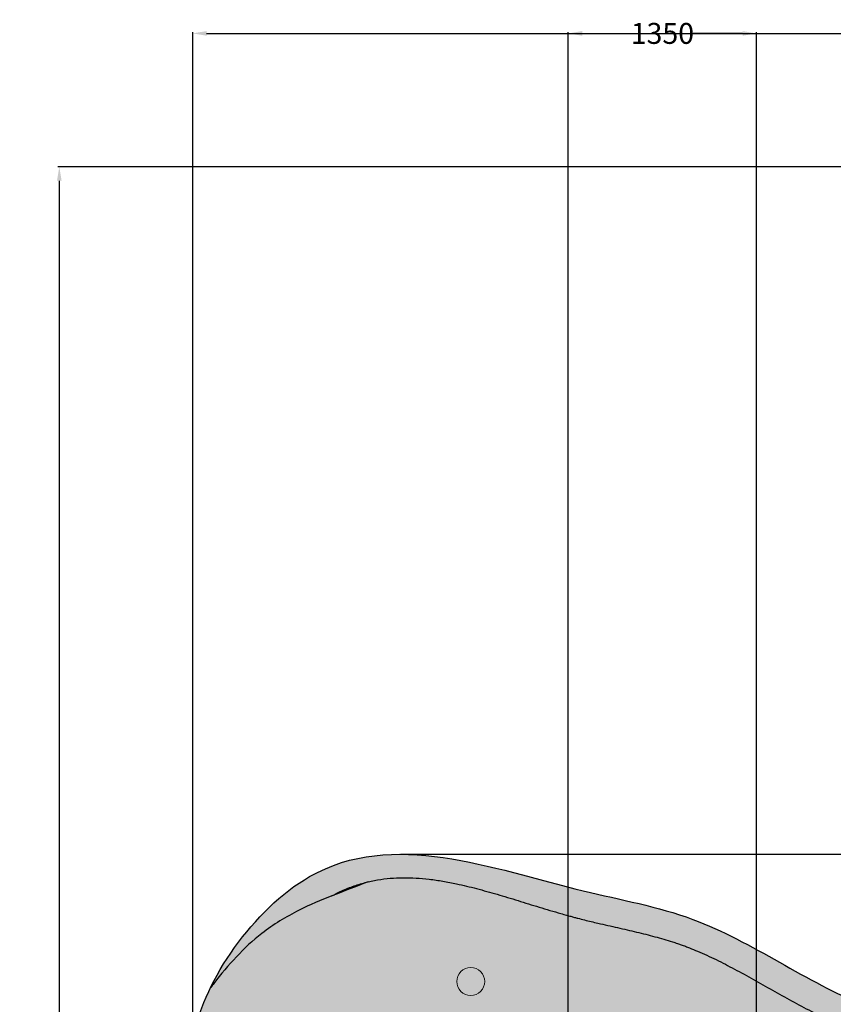
# Model space of a CAD drawing. Units: millimetres. Extents: x 11032 to 26788, y 3406 to 24505.
# Tile 75 of 78: x 11061 to 16895, y 17443 to 24505. Entities that reach past the tile are written whole.
import ezdxf

# ---------------------------------------------------------------- set-up
doc = ezdxf.new("R2010")
doc.units = ezdxf.units.MM
doc.header["$MEASUREMENT"] = 0
for name, color, linetype, lineweight in [('A-ANNO-DIMS', 2, 'Continuous', 18), ('A-ROOF', 7, 'Continuous', 30), ('E-LITE', 7, 'Continuous', 18), ('E-LITE-PATT', 7, 'Continuous', 13)]:
    doc.layers.add(name, color=color, linetype=linetype, lineweight=lineweight)
doc.layers.add('A-ROOF-PATT', color=9, linetype='Continuous', lineweight=13, true_color=0xc7c8ca)
doc.styles.get("Standard").update_dxf_attribs({"font": 'arial.ttf'})
doc.dimstyles.get("Standard").update_dxf_attribs({"dimtxt": 150, "dimasz": 100, "dimexe": 10, "dimexo": 5, "dimgap": 5, "dimtad": 0, "dimtih": 1, "dimtoh": 1, "dimdec": 0, "dimzin": 0, "dimdsep": 46, "dimtxsty": 'Standard', "dimcen": 0.09, "dimadec": 0, "dimazin": 0, "dimtfac": 1, "dimtdec": 0, "dimtofl": 0, "dimtmove": 0, "dimatfit": 3, "dimfxl": 1, "dimtolj": 1, "dimtzin": 0, "dimarcsym": 0})

# ---------------------------------------------------------------- blocks, each defined once
blk = doc.blocks.new('RECESSED-LIGHT-200')
blk.add_circle((100, 100), 100)
blk = doc.blocks.new('*D24')
at = {"layer": 'A-ANNO-DIMS', "color": 0, "lineweight": -2, "transparency": 16777216}
for p, q in [((13210.2, 17163), (13110.2, 17163)), ((13310.2, 17138), (13310.2, 17173)), ((13510.2, 17138), (13510.2, 17173)), ((13610.2, 17163), (13710.2, 17163))]:
    blk.add_line(p, q, dxfattribs=at)
at = {"layer": 'A-ANNO-DIMS', "color": 0, "transparency": 16777216}
for points in [[(13210.2, 17179.6), (13210.2, 17146.3), (13310.2, 17163)], [(13610.2, 17179.6), (13610.2, 17146.3), (13510.2, 17163)]]:
    blk.add_solid(points, dxfattribs=at)
at = {"layer": 'Defpoints', "color": 0, "transparency": 16777216}
for p in [(13510.2, 17163), (13310.2, 17133), (13510.2, 17133)]:
    blk.add_point(p, dxfattribs=at)
at = {"layer": 'A-ANNO-DIMS', "color": 0, "transparency": 16777216, "insert": (15077.8, 17163), "char_height": 150, "attachment_point": 5}
blk.add_mtext('\\A1;RECESSED LIGHT 200 TYP.', dxfattribs=at)
blk = doc.blocks.new('*D36')
at = {"layer": 'A-ANNO-DIMS', "color": 0, "lineweight": -2, "transparency": 16777216}
for p, q in [((12301.3, 17115.9), (12301.3, 24416.9)), ((12401.3, 24406.9), (18569.2, 24406.9)), ((25297.4, 24406.9), (19129.5, 24406.9)), ((25397.4, 4466.4), (25397.4, 24416.9))]:
    blk.add_line(p, q, dxfattribs=at)
at = {"layer": 'A-ANNO-DIMS', "color": 0, "transparency": 16777216}
for points in [[(12401.3, 24423.5), (12401.3, 24390.2), (12301.3, 24406.9)], [(25297.4, 24423.5), (25297.4, 24390.2), (25397.4, 24406.9)]]:
    blk.add_solid(points, dxfattribs=at)
at = {"layer": 'Defpoints', "color": 0, "transparency": 16777216}
for p in [(25397.4, 24406.9), (12301.3, 17110.9), (25397.4, 4461.4)]:
    blk.add_point(p, dxfattribs=at)
at = {"layer": 'A-ANNO-DIMS', "color": 0, "transparency": 16777216, "insert": (18849.3, 24406.9), "char_height": 150, "attachment_point": 5}
blk.add_mtext('\\A1;13096', dxfattribs=at)
blk = doc.blocks.new('*D37')
at = {"layer": 'A-ANNO-DIMS', "color": 0, "lineweight": -2, "transparency": 16777216}
for p, q in [((18087.7, 23450.4), (11334.8, 23450.4)), ((11344.8, 23350.4), (11344.8, 14037.5)), ((11344.8, 4561.4), (11344.8, 13874.3)), ((12927.7, 4461.4), (11334.8, 4461.4))]:
    blk.add_line(p, q, dxfattribs=at)
at = {"layer": 'A-ANNO-DIMS', "color": 0, "transparency": 16777216}
for points in [[(11328.1, 23350.4), (11361.4, 23350.4), (11344.8, 23450.4)], [(11328.1, 4561.4), (11361.4, 4561.4), (11344.8, 4461.4)]]:
    blk.add_solid(points, dxfattribs=at)
at = {"layer": 'Defpoints', "color": 0, "transparency": 16777216}
for p in [(11344.8, 23450.4), (18092.7, 23450.4), (12932.7, 4461.4)]:
    blk.add_point(p, dxfattribs=at)
at = {"layer": 'A-ANNO-DIMS', "color": 0, "transparency": 16777216, "insert": (11344.8, 13955.9), "char_height": 150, "attachment_point": 5}
blk.add_mtext('\\A1;18989', dxfattribs=at)
blk = doc.blocks.new('*D45')
at = {"layer": 'A-ANNO-DIMS', "color": 0, "lineweight": -2, "transparency": 16777216}
for p, q in [((13792.4, 18518.9), (26363.9, 18518.9)), ((26353.9, 18418.9), (26353.9, 17450.3)), ((26353.9, 16318.4), (26353.9, 17287)), ((22902.4, 16218.4), (26363.9, 16218.4))]:
    blk.add_line(p, q, dxfattribs=at)
at = {"layer": 'A-ANNO-DIMS', "color": 0, "transparency": 16777216}
for points in [[(26337.2, 18418.9), (26370.6, 18418.9), (26353.9, 18518.9)], [(26337.2, 16318.4), (26370.6, 16318.4), (26353.9, 16218.4)]]:
    blk.add_solid(points, dxfattribs=at)
at = {"layer": 'Defpoints', "color": 0, "transparency": 16777216}
for p in [(13787.4, 18518.9), (26353.9, 18518.9), (22897.4, 16218.4)]:
    blk.add_point(p, dxfattribs=at)
at = {"layer": 'A-ANNO-DIMS', "color": 0, "transparency": 16777216, "insert": (26353.9, 17368.7), "char_height": 150, "attachment_point": 5}
blk.add_mtext('\\A1;2300.5', dxfattribs=at)
blk = doc.blocks.new('*D46')
at = {"layer": 'A-ANNO-DIMS', "color": 0, "lineweight": -2, "transparency": 16777216}
for p, q in [((18497.2, 21762.9), (26363.9, 21762.9)), ((26353.9, 21662.9), (26353.9, 20222.6)), ((26353.9, 18618.9), (26353.9, 20059.3)), ((13792.4, 18518.9), (26363.9, 18518.9))]:
    blk.add_line(p, q, dxfattribs=at)
at = {"layer": 'A-ANNO-DIMS', "color": 0, "transparency": 16777216}
for points in [[(26337.2, 21662.9), (26370.6, 21662.9), (26353.9, 21762.9)], [(26337.2, 18618.9), (26370.6, 18618.9), (26353.9, 18518.9)]]:
    blk.add_solid(points, dxfattribs=at)
at = {"layer": 'Defpoints', "color": 0, "transparency": 16777216}
for p in [(18492.2, 21762.9), (26353.9, 21762.9), (13787.4, 18518.9)]:
    blk.add_point(p, dxfattribs=at)
at = {"layer": 'A-ANNO-DIMS', "color": 0, "transparency": 16777216, "insert": (26353.9, 20140.9), "char_height": 150, "attachment_point": 5}
blk.add_mtext('\\A1;3244', dxfattribs=at)
blk = doc.blocks.new('*D57')
at = {"layer": 'A-ANNO-DIMS', "color": 0, "lineweight": -2, "transparency": 16777216}
for p, q in [((14994.7, 7266.4), (14994.7, 24416.9)), ((15094.7, 24406.9), (17716, 24406.9)), ((20794.7, 24406.9), (18173.4, 24406.9)), ((20894.7, 7266.4), (20894.7, 24416.9))]:
    blk.add_line(p, q, dxfattribs=at)
at = {"layer": 'A-ANNO-DIMS', "color": 0, "transparency": 16777216}
for points in [[(15094.7, 24423.5), (15094.7, 24390.2), (14994.7, 24406.9)], [(20794.7, 24423.5), (20794.7, 24390.2), (20894.7, 24406.9)]]:
    blk.add_solid(points, dxfattribs=at)
at = {"layer": 'Defpoints', "color": 0, "transparency": 16777216}
for p in [(20894.7, 24406.9), (14994.7, 7261.4), (20894.7, 7261.4)]:
    blk.add_point(p, dxfattribs=at)
at = {"layer": 'A-ANNO-DIMS', "color": 0, "transparency": 16777216, "insert": (17944.7, 24406.9), "char_height": 150, "attachment_point": 5}
blk.add_mtext('\\A1;5900', dxfattribs=at)
blk = doc.blocks.new('*D60')
at = {"layer": 'A-ANNO-DIMS', "color": 0, "lineweight": -2, "transparency": 16777216}
for p, q in [((14994.7, 7266.4), (14994.7, 24416.9)), ((15094.7, 24406.9), (15448, 24406.9)), ((16244.7, 24406.9), (15891.4, 24406.9)), ((16344.7, 7266.4), (16344.7, 24416.9))]:
    blk.add_line(p, q, dxfattribs=at)
at = {"layer": 'A-ANNO-DIMS', "color": 0, "transparency": 16777216}
for points in [[(15094.7, 24423.5), (15094.7, 24390.2), (14994.7, 24406.9)], [(16244.7, 24423.5), (16244.7, 24390.2), (16344.7, 24406.9)]]:
    blk.add_solid(points, dxfattribs=at)
at = {"layer": 'Defpoints', "color": 0, "transparency": 16777216}
for p in [(16344.7, 24406.9), (14994.7, 7261.4), (16344.7, 7261.4)]:
    blk.add_point(p, dxfattribs=at)
at = {"layer": 'A-ANNO-DIMS', "color": 0, "transparency": 16777216, "insert": (15669.7, 24406.9), "char_height": 150, "attachment_point": 5}
blk.add_mtext('\\A1;1350', dxfattribs=at)

msp = doc.modelspace()

# ---------------------------------------------------------------- hatches: boundary and pattern name
at = {"layer": 'A-ROOF-PATT'}
h = msp.add_hatch(color=256, dxfattribs=at)
edge = h.paths.add_edge_path()
edge.add_spline(control_points=[(17532.827, 17324.837), (17391.335, 17349.016), (16840.872, 17494.912), (16080.055, 18069.544), (14738.803, 18299.641), (13382.429, 18838.336), (12580.532, 17870.207), (12430.422, 17563.822)], knot_values=[2977.60279446, 2977.60279446, 2977.60279446, 2977.60279446, 3438.18406011, 4811.64630219, 5622.86754827, 7588.02881883, 8560.66857913, 8560.66857913, 8560.66857913, 8560.66857913], degree=3, periodic=0)
edge.add_spline(control_points=[(12430.422, 17563.822), (12437.904, 17573.36), (12445.386, 17582.899), (12452.869, 17592.437), (12452.869, 17592.438), (12452.869, 17592.438), (12452.869, 17592.438)], knot_values=[1408.56413798, 1408.56413798, 1408.56413798, 1408.56413798, 1444.85989, 1444.85989, 1444.85989, 1444.86011829, 1444.86011829, 1444.86011829, 1444.86011829], degree=3, periodic=0)
edge.add_spline(control_points=[(12452.869, 17592.438), (12555.432, 17723.185), (12736.557, 17929.686), (13044.86, 18114.643), (13219.943, 18189.644), (13299.92, 18220.646)], knot_values=[339.31824597, 339.31824597, 339.31824597, 339.31824597, 836.83499673, 1151.25129334, 1408.56413798, 1408.56413798, 1408.56413798, 1408.56413798], degree=3, periodic=0)
edge.add_spline(control_points=[(13299.92, 18220.646), (13299.998, 18220.689), (13300.077, 18220.732), (13319.738, 18231.488), (13339.24, 18241.402), (13388.645, 18264.703), (13418.466, 18277.069), (13478.019, 18298.648), (13507.751, 18307.861), (13544.561, 18317.488), (13551.584, 18319.245), (13558.612, 18320.924)], knot_values=[3783.89509717, 3783.89509717, 3783.89509717, 3783.89509717, 3784.1737101, 3784.1737101, 3853.4666747, 3853.4666747, 3960.24019172, 3960.24019172, 4067.01370874, 4067.01370874, 4092.17446487, 4092.17446487, 4092.17446487, 4092.17446487], degree=3, periodic=0)
edge.add_spline(control_points=[(13558.612, 18320.924), (13581.407, 18326.373), (13604.25, 18331.007), (13657.184, 18339.957), (13687.338, 18343.732), (13748.098, 18348.892), (13778.704, 18350.276), (13840.46, 18350.833), (13871.609, 18350.005), (13934.496, 18346.313), (13966.232, 18343.449), (14030.297, 18335.871), (14062.625, 18331.158), (14127.853, 18320.088), (14160.753, 18313.73), (14241.357, 18296.556), (14289.343, 18284.997), (14386.31, 18259.688), (14435.291, 18245.941), (14534.161, 18217.034), (14584.049, 18201.875), (14684.682, 18170.964), (14735.427, 18155.212), (14837.763, 18123.971), (14889.354, 18108.482), (14954.971, 18089.677), (14968.586, 18085.823), (14992.391, 18079.184), (15002.566, 18076.376), (15021.739, 18071.153), (15030.731, 18068.729), (15047.707, 18064.21), (15055.694, 18062.106), (15079.815, 18055.825), (15095.905, 18051.728), (15143.966, 18039.717), (15175.729, 18032.084), (15254.84, 18013.501), (15301.798, 18002.866), (15394.186, 17981.845), (15439.615, 17971.459), (15528.833, 17950.135), (15572.62, 17939.197), (15658.477, 17916.021), (15700.546, 17903.785), (15753.633, 17886.734), (15765.446, 17882.835), (15786.574, 17875.653), (15795.915, 17872.404), (15810.108, 17867.349), (15814.99, 17865.588), (15824.736, 17862.029), (15829.611, 17860.226), (15844.241, 17854.75), (15854.002, 17851.008), (15883.312, 17839.521), (15902.885, 17831.512), (15966.355, 17804.548), (16010.39, 17784.302), (16098.838, 17741.267), (16143.25, 17718.478), (16232.497, 17671.098), (16277.332, 17646.507), (16367.515, 17596.295), (16412.862, 17570.676), (16504.202, 17519.209), (16550.194, 17493.362), (16643.009, 17442.263), (16689.831, 17417.011), (16756.517, 17382.472), (16775.937, 17372.58), (16795.455, 17362.84)], knot_values=[4092.17446487, 4092.17446487, 4092.17446487, 4092.17446487, 4173.78722577, 4173.78722577, 4280.56074279, 4280.56074279, 4387.33425981, 4387.33425981, 4494.10777683, 4494.10777683, 4600.88129386, 4600.88129386, 4707.65481088, 4707.65481088, 4814.4283279, 4814.4283279, 4967.12624049, 4967.12624049, 5119.82415308, 5119.82415308, 5272.52206566, 5272.52206566, 5425.21997825, 5425.21997825, 5577.91789084, 5577.91789084, 5617.78533194, 5617.78533194, 5647.46484794, 5647.46484794, 5673.61102495, 5673.61102495, 5696.74760695, 5696.74760695, 5743.68189033, 5743.68189033, 5837.55045709, 5837.55045709, 5979.72610459, 5979.72610459, 6121.90175208, 6121.90175208, 6264.07739957, 6264.07739957, 6406.25304706, 6406.25304706, 6447.25858494, 6447.25858494, 6480.04208821, 6480.04208821, 6497.30770621, 6497.30770621, 6514.5733242, 6514.5733242, 6549.10456019, 6549.10456019, 6618.16703217, 6618.16703217, 6772.66101707, 6772.66101707, 6927.15500198, 6927.15500198, 7081.64898689, 7081.64898689, 7236.1429718, 7236.1429718, 7390.6369567, 7390.6369567, 7545.13094161, 7545.13094161, 7608.19928683, 7608.19928683, 7608.19928683, 7608.19928683], degree=3, periodic=0)
edge.add_spline(control_points=[(16795.455, 17362.84), (16814.335, 17349.456), (16832.897, 17336.263), (16873.225, 17307.197), (16894.778, 17291.386), (16936.221, 17259.941), (16956.11, 17244.308), (16993.863, 17213.094), (17011.726, 17197.514), (17041.993, 17169.265), (17054.791, 17156.601), (17078.762, 17131.225), (17089.933, 17118.516), (17110.618, 17092.991), (17120.131, 17080.178), (17130.17, 17065.264), (17131.487, 17063.277), (17133.77, 17059.776), (17134.746, 17058.261), (17136.69, 17055.205), (17137.657, 17053.668), (17140.539, 17049.025), (17142.438, 17045.89), (17148.068, 17036.367), (17151.732, 17029.859), (17163.03, 17008.788), (17170.335, 16993.646), (17184.087, 16961.978), (17190.534, 16945.453), (17202.562, 16911.165), (17208.142, 16893.402), (17218.448, 16856.821), (17223.173, 16838.003), (17231.801, 16799.51), (17235.705, 16779.837), (17241.533, 16746.739), (17243.676, 16733.5), (17247.718, 16706.37), (17249.608, 16692.472), (17252.066, 16672.69), (17252.761, 16666.875), (17254.1, 16655.226), (17254.744, 16649.4), (17256.596, 16631.917), (17257.727, 16620.254), (17260.823, 16585.238), (17262.489, 16561.858), (17266.551, 16488.654), (17267.658, 16438.661), (17267.349, 16375.228), (17267.193, 16362.07), (17266.95, 16348.891)], knot_values=[15.11304723, 15.11304723, 15.11304723, 15.11304723, 82.69951457, 82.69951457, 165.39902914, 165.39902914, 248.09854371, 248.09854371, 330.79805828, 330.79805828, 397.94194582, 397.94194582, 465.08583335, 465.08583335, 532.22972088, 532.22972088, 542.53374101, 542.53374101, 550.35681582, 550.35681582, 558.17989062, 558.17989062, 573.82604024, 573.82604024, 605.11833946, 605.11833946, 672.76406143, 672.76406143, 740.4097834, 740.4097834, 808.05550537, 808.05550537, 875.70122735, 875.70122735, 943.34694932, 943.34694932, 987.66134917, 987.66134917, 1033.41216123, 1033.41216123, 1052.38508762, 1052.38508762, 1071.35801402, 1071.35801402, 1109.30386682, 1109.30386682, 1185.19557241, 1185.19557241, 1346.44190265, 1346.44190265, 1388.55866312, 1388.55866312, 1388.55866312, 1388.55866312], degree=3, periodic=0)
edge.add_spline(control_points=[(17266.95, 16348.891), (17266.95, 16348.891), (17266.95, 16348.891), (17266.95, 16348.891), (17253.182, 15602.417), (17239.414, 14855.943), (17225.646, 14109.469)], knot_values=[1388.55866312, 1388.55866312, 1388.55866312, 1388.55866312, 1388.55896543, 1388.55896543, 1388.55896543, 3774.07676609, 3774.07676609, 3774.07676609, 3774.07676609], degree=3, periodic=0)
edge.add_spline(control_points=[(17225.646, 14109.469), (17226.198, 14109.827), (17226.748, 14110.185), (17242.065, 14120.191), (17255.956, 14130.116), (17274.422, 14144.286), (17279.609, 14148.386), (17284.686, 14152.511)], knot_values=[1926.3423968, 1926.3423968, 1926.3423968, 1926.3423968, 1927.31672898, 1927.31672898, 1953.51217613, 1953.51217613, 1964.07323478, 1964.07323478, 1964.07323478, 1964.07323478], degree=3, periodic=0)
edge.add_spline(control_points=[(17284.686, 14152.511), (17315.791, 14194.761), (17384.413, 14446.273), (17407.128, 14793.401), (17407.093, 15295.84), (17423.274, 15626.362), (17415.601, 15782.507)], knot_values=[0, 0, 0, 0, 163.25546741, 619.22967667, 1171.8624483, 1621.63555623, 1621.63555623, 1621.63555623, 1621.63555623], degree=3, periodic=0)
edge.add_spline(control_points=[(17415.601, 15782.507), (17438.21, 16077.57), (17410.495, 16533.484), (17390.893, 17030.649), (17301.082, 17169.349)], knot_values=[543.97847526, 543.97847526, 543.97847526, 543.97847526, 1452.98527668, 1960.01149261, 1960.01149261, 1960.01149261, 1960.01149261], degree=3, periodic=0)
edge.add_spline(control_points=[(17301.082, 17169.349), (17346.58, 17157.64), (17392.235, 17147.336), (17467.161, 17132.609), (17496.336, 17127.412), (17525.58, 17122.709)], knot_values=[8131.59393903, 8131.59393903, 8131.59393903, 8131.59393903, 8269.73492727, 8269.73492727, 8357.5016646, 8357.5016646, 8357.5016646, 8357.5016646], degree=3, periodic=0)
edge.add_line((17525.58, 17122.709), (17532.827, 17324.837))
edge = h.paths.add_edge_path(flags=17)
edge.add_spline(control_points=[(13340.537, 14602.706), (13316.172, 14726.456), (13323.666, 14932.342), (13637.836, 15081.117), (13863.248, 15171.051), (14002.1, 15224.503), (14058.539, 15244.876)], knot_values=[680.89318617, 680.89318617, 680.89318617, 680.89318617, 1033.47282894, 1337.40083264, 1604.72142636, 1784.29447217, 1784.29447217, 1784.29447217, 1784.29447217], degree=3, periodic=0)
edge.add_spline(control_points=[(14058.539, 15244.876), (14058.289, 15275.236), (14057.634, 15305.434), (14055.312, 15376.527), (14053.359, 15417.248), (14048.642, 15497.048), (14045.89, 15536.143), (14042.888, 15574.619)], knot_values=[6573.10654186, 6573.10654186, 6573.10654186, 6573.10654186, 6636.73300118, 6636.73300118, 6723.88905466, 6723.88905466, 6809.63287714, 6809.63287714, 6809.63287714, 6809.63287714], degree=3, periodic=0)
edge.add_spline(control_points=[(14042.888, 15574.619), (13546.54, 15403.221), (13074.735, 15143.241), (13277.36, 14695.339), (13340.537, 14602.706)], knot_values=[503.79257829, 503.79257829, 503.79257829, 503.79257829, 1728.17876056, 2051.34843998, 2051.34843998, 2051.34843998, 2051.34843998], degree=3, periodic=0)
h = msp.add_hatch(color=256, dxfattribs=at)
h.set_gradient(color1=(254, 234, 185), color2=(254, 204, 102), name='HEMISPHERICAL')
edge = h.paths.add_edge_path()
edge.add_line((15084.393, 17001.32), (15284.393, 17051.32))
edge.add_line((15284.393, 17051.32), (15470.537, 16752.334))
edge.add_spline(control_points=[(15470.537, 16752.334), (15683.311, 16831.508), (16106.827, 16912.335), (16625.609, 16876.997), (17083.498, 16357.78), (17257.801, 16180.113)], knot_values=[0, 0, 0, 0, 655.29363337, 1252.01578382, 1989.61628586, 1989.61628586, 1989.61628586, 1989.61628586], degree=3, periodic=0)
edge.add_spline(control_points=[(17257.801, 16180.113), (17260.851, 16236.372), (17263.9, 16292.632), (17266.95, 16348.891)], knot_values=[1132.9967717, 1132.9967717, 1132.9967717, 1132.9967717, 1198.04642249, 1198.04642249, 1198.04642249, 1198.04642249], degree=3, periodic=0)
edge.add_spline(control_points=[(17266.95, 16348.891), (17267.193, 16362.07), (17267.349, 16375.228), (17267.658, 16438.661), (17266.551, 16488.654), (17262.489, 16561.858), (17260.823, 16585.238), (17257.727, 16620.254), (17256.596, 16631.917), (17254.744, 16649.4), (17254.1, 16655.226), (17252.761, 16666.875), (17252.066, 16672.69), (17249.608, 16692.472), (17247.718, 16706.37), (17243.676, 16733.5), (17241.533, 16746.739), (17235.705, 16779.837), (17231.801, 16799.51), (17223.173, 16838.003), (17218.448, 16856.821), (17208.142, 16893.402), (17202.562, 16911.165), (17190.534, 16945.453), (17184.087, 16961.978), (17170.335, 16993.646), (17163.03, 17008.788), (17151.732, 17029.859), (17148.068, 17036.367), (17142.438, 17045.89), (17140.539, 17049.025), (17137.657, 17053.668), (17136.69, 17055.205), (17134.746, 17058.261), (17133.77, 17059.776), (17131.487, 17063.277), (17130.17, 17065.264), (17120.131, 17080.178), (17110.618, 17092.991), (17089.933, 17118.516), (17078.762, 17131.225), (17054.791, 17156.601), (17041.993, 17169.265), (17011.726, 17197.514), (16993.863, 17213.094), (16956.11, 17244.308), (16936.221, 17259.941), (16894.778, 17291.386), (16873.225, 17307.197), (16832.897, 17336.263), (16814.335, 17349.456), (16795.455, 17362.84)], knot_values=[15.11304723, 15.11304723, 15.11304723, 15.11304723, 57.2298077, 57.2298077, 218.47613793, 218.47613793, 294.36784353, 294.36784353, 332.31369632, 332.31369632, 351.28662272, 351.28662272, 370.25954912, 370.25954912, 416.01036118, 416.01036118, 460.32476103, 460.32476103, 527.970483, 527.970483, 595.61620497, 595.61620497, 663.26192694, 663.26192694, 730.90764891, 730.90764891, 798.55337089, 798.55337089, 829.84567011, 829.84567011, 845.49181972, 845.49181972, 853.31489453, 853.31489453, 861.13796933, 861.13796933, 871.44198947, 871.44198947, 938.585877, 938.585877, 1005.72976453, 1005.72976453, 1072.87365206, 1072.87365206, 1155.57316663, 1155.57316663, 1238.2726812, 1238.2726812, 1320.97219578, 1320.97219578, 1388.55866312, 1388.55866312, 1388.55866312, 1388.55866312], degree=3, periodic=0)
edge.add_spline(control_points=[(16795.455, 17362.84), (16775.937, 17372.58), (16756.517, 17382.472), (16689.831, 17417.011), (16643.009, 17442.263), (16550.194, 17493.362), (16504.202, 17519.209), (16412.862, 17570.676), (16367.515, 17596.295), (16277.332, 17646.507), (16232.497, 17671.098), (16143.25, 17718.478), (16098.838, 17741.267), (16010.39, 17784.302), (15966.355, 17804.548), (15902.885, 17831.512), (15883.312, 17839.521), (15854.002, 17851.008), (15844.241, 17854.75), (15829.611, 17860.226), (15824.736, 17862.029), (15814.99, 17865.588), (15810.108, 17867.349), (15795.915, 17872.404), (15786.574, 17875.653), (15765.446, 17882.835), (15753.633, 17886.734), (15700.546, 17903.785), (15658.477, 17916.021), (15572.62, 17939.197), (15528.833, 17950.135), (15439.615, 17971.459), (15394.186, 17981.845), (15301.798, 18002.866), (15254.84, 18013.501), (15175.729, 18032.084), (15143.966, 18039.717), (15095.905, 18051.728), (15079.815, 18055.825), (15055.694, 18062.106), (15047.707, 18064.21), (15030.731, 18068.729), (15021.739, 18071.153), (15002.566, 18076.376), (14992.391, 18079.184), (14968.586, 18085.823), (14954.971, 18089.677), (14889.354, 18108.482), (14837.763, 18123.971), (14735.427, 18155.212), (14684.682, 18170.964), (14584.049, 18201.875), (14534.161, 18217.034), (14435.291, 18245.941), (14386.31, 18259.688), (14289.343, 18284.997), (14241.357, 18296.556), (14160.753, 18313.73), (14127.853, 18320.088), (14062.625, 18331.158), (14030.297, 18335.871), (13966.232, 18343.449), (13934.496, 18346.313), (13871.609, 18350.005), (13840.46, 18350.833), (13778.704, 18350.276), (13748.098, 18348.892), (13687.338, 18343.732), (13657.184, 18339.957), (13604.25, 18331.007), (13581.407, 18326.373), (13558.612, 18320.924)], knot_values=[4092.17446487, 4092.17446487, 4092.17446487, 4092.17446487, 4155.24281009, 4155.24281009, 4309.736795, 4309.736795, 4464.2307799, 4464.2307799, 4618.72476481, 4618.72476481, 4773.21874972, 4773.21874972, 4927.71273463, 4927.71273463, 5082.20671953, 5082.20671953, 5151.26919151, 5151.26919151, 5185.8004275, 5185.8004275, 5203.0660455, 5203.0660455, 5220.33166349, 5220.33166349, 5253.11516676, 5253.11516676, 5294.12070464, 5294.12070464, 5436.29635213, 5436.29635213, 5578.47199962, 5578.47199962, 5720.64764711, 5720.64764711, 5862.82329461, 5862.82329461, 5956.69186137, 5956.69186137, 6003.62614475, 6003.62614475, 6026.76272675, 6026.76272675, 6052.90890376, 6052.90890376, 6082.58841976, 6082.58841976, 6122.45586086, 6122.45586086, 6275.15377345, 6275.15377345, 6427.85168604, 6427.85168604, 6580.54959862, 6580.54959862, 6733.24751121, 6733.24751121, 6885.9454238, 6885.9454238, 6992.71894082, 6992.71894082, 7099.49245784, 7099.49245784, 7206.26597487, 7206.26597487, 7313.03949189, 7313.03949189, 7419.81300891, 7419.81300891, 7526.58652593, 7526.58652593, 7608.19928683, 7608.19928683, 7608.19928683, 7608.19928683], degree=3, periodic=0)
edge.add_spline(control_points=[(13558.612, 18320.924), (13472.381, 18287.498), (13386.15, 18254.072), (13299.92, 18220.646), (13299.92, 18220.646), (13299.92, 18220.646), (13299.92, 18220.646)], knot_values=[61.88324569, 61.88324569, 61.88324569, 61.88324569, 339.3179746, 339.3179746, 339.3179746, 339.31824597, 339.31824597, 339.31824597, 339.31824597], degree=3, periodic=0)
edge.add_spline(control_points=[(13299.92, 18220.646), (13219.943, 18189.644), (13044.86, 18114.643), (12736.557, 17929.686), (12555.432, 17723.185), (12452.869, 17592.438)], knot_values=[339.31824597, 339.31824597, 339.31824597, 339.31824597, 596.63109061, 911.04738723, 1408.56413798, 1408.56413798, 1408.56413798, 1408.56413798], degree=3, periodic=0)
edge.add_spline(control_points=[(12452.869, 17592.438), (12452.869, 17592.438), (12452.869, 17592.438), (12452.869, 17592.437), (12445.386, 17582.899), (12437.904, 17573.36), (12430.422, 17563.822)], knot_values=[1408.56413798, 1408.56413798, 1408.56413798, 1408.56413798, 1408.56436627, 1408.56436627, 1408.56436627, 1444.86011829, 1444.86011829, 1444.86011829, 1444.86011829], degree=3, periodic=0)
edge.add_spline(control_points=[(12430.422, 17563.822), (12373.797, 17448.248), (12157.302, 16836.764), (12751.985, 16393.69), (13424.325, 15907.903), (14042.888, 15574.619)], knot_values=[0, 0, 0, 0, 366.89930338, 1975.59410824, 2977.60279446, 2977.60279446, 2977.60279446, 2977.60279446], degree=3, periodic=0)
edge.add_spline(control_points=[(14042.888, 15574.619), (14042.839, 15575.252), (14042.789, 15575.886), (14039.681, 15615.607), (14036.366, 15654.052), (14029.551, 15729.305), (14026.05, 15766.114), (14019.175, 15837.686), (14015.8, 15872.45), (13903.823, 16338.596)], knot_values=[6310.22615039, 6310.22615039, 6310.22615039, 6310.22615039, 6311.63838141, 6311.63838141, 6398.79443489, 6398.79443489, 6485.95048837, 6485.95048837, 6573.10654186, 6573.10654186, 6573.10654186, 6573.10654186], degree=3, periodic=0)
edge.add_spline(control_points=[(13903.823, 16338.596), (14237.315, 16236.889), (14456.623, 16167.555), (14614.196, 16115.84)], knot_values=[0, 0, 0, 0, 202.98534191, 202.98534191, 202.98534191, 202.98534191], degree=3, periodic=0)
edge.add_spline(control_points=[(14614.196, 16115.84), (14663.209, 16178.992), (14799.965, 16341.237), (14969.915, 16481.426), (15084.393, 16556.825)], knot_values=[2405.03450449, 2405.03450449, 2405.03450449, 2405.03450449, 2644.88269663, 3039.27072715, 3039.27072715, 3039.27072715, 3039.27072715], degree=3, periodic=0)
edge.add_line((15084.393, 16556.825), (15084.393, 17001.32))
h.paths.add_polyline_path([(14195.599, 17606.181, -1), (14395.599, 17606.181, -1)], flags=16)
h.paths.add_polyline_path([(13310.178, 17032.97, -1), (13510.178, 17032.97, -1)], flags=16)
at = {"layer": 'E-LITE-PATT'}
h = msp.add_hatch(color=256, dxfattribs=at)
h.paths.add_polyline_path([(13510.178, 17032.97, 1), (13310.178, 17032.97, 1)])
h.paths.add_polyline_path([(14395.599, 17606.181, 1), (14195.599, 17606.181, 1)])
h.paths.add_polyline_path([(16625.717, 16408.125, 1), (16475.717, 16408.125, 1)])
h.paths.add_polyline_path([(16348.536, 16037.613, 1), (16198.536, 16037.613, 1)])
h.paths.add_polyline_path([(16624.605, 15622.642, 1), (16474.605, 15622.642, 1)])
edge = h.paths.add_edge_path()
edge.add_spline(control_points=[(17236.862, 15254.714), (17229.535, 15256.737), (17222.182, 15258.759), (17198.292, 15265.245), (17181.692, 15269.627), (17148.526, 15277.734), (17131.961, 15281.46), (17101.972, 15287.211), (17088.519, 15289.422), (17061.76, 15292.783), (17048.453, 15293.935), (17024.904, 15294.713), (17014.631, 15294.619), (16994.186, 15293.334), (16984.013, 15292.142), (16965.985, 15288.78), (16958.1, 15286.873), (16942.515, 15282.052), (16934.816, 15279.138), (16919.756, 15272.176), (16912.397, 15268.127), (16898.232, 15258.834), (16891.428, 15253.591), (16878.593, 15241.952), (16872.565, 15235.558), (16864.978, 15226.136), (16863.017, 15223.558), (16859.188, 15218.226), (16857.321, 15215.468), (16853.744, 15209.868), (16852.029, 15207.021), (16847.092, 15198.353), (16844.079, 15192.402), (16838.565, 15180.211), (16836.065, 15173.969), (16830.486, 15158.22), (16827.696, 15148.567), (16823.186, 15128.868), (16821.467, 15118.823), (16819.162, 15098.483), (16818.576, 15088.188), (16818.649, 15067.496), (16819.308, 15057.097), (16822.047, 15036.354), (16824.126, 15026.008), (16829.289, 15007.911), (16832.033, 15000.109), (16838.658, 14984.798), (16842.539, 14977.287), (16849.83, 14965.576), (16852.841, 14961.219), (16856.103, 14956.992)], knot_values=[9.66395345, 9.66395345, 9.66395345, 9.66395345, 27.53412528, 27.53412528, 67.58923678, 67.58923678, 107.64434828, 107.64434828, 140.47601017, 140.47601017, 173.30767206, 173.30767206, 198.91119899, 198.91119899, 224.51472592, 224.51472592, 244.64945969, 244.64945969, 264.78419346, 264.78419346, 284.91892722, 284.91892722, 305.05366099, 305.05366099, 325.18839476, 325.18839476, 332.50248756, 332.50248756, 339.93943037, 339.93943037, 347.37637318, 347.37637318, 362.25025881, 362.25025881, 377.12414443, 377.12414443, 399.05652947, 399.05652947, 420.9889145, 420.9889145, 442.92129954, 442.92129954, 464.85368458, 464.85368458, 486.78606961, 486.78606961, 503.69207808, 503.69207808, 520.59808656, 520.59808656, 530.96929985, 530.96929985, 530.96929985, 530.96929985], degree=3, periodic=0)
edge.add_spline(control_points=[(16856.103, 14956.992), (16835.647, 14956.617), (16813.531, 14956.412), (16766.918, 14956.255), (16742.419, 14956.302), (16691.933, 14956.554), (16665.945, 14956.759), (16622.516, 14957.149), (16605.253, 14957.316), (16587.978, 14957.484)], knot_values=[872.21819251, 872.21819251, 872.21819251, 872.21819251, 915.29845126, 915.29845126, 958.37871, 958.37871, 1001.45896875, 1001.45896875, 1029.52650638, 1029.52650638, 1029.52650638, 1029.52650638], degree=3, periodic=0)
edge.add_line((16587.978, 14957.484), (16619.296, 14907.181))
edge.add_spline(control_points=[(16619.296, 14907.181), (16852.686, 14904.98), (17116.098, 14904.13), (16849.359, 14976.117), (16870.954, 15304.114), (17098.337, 15241.178), (17235.385, 15203.245)], knot_values=[0, 0, 0, 0, 380.18823763, 455.22852006, 676.53552898, 1012.28787348, 1012.28787348, 1012.28787348, 1012.28787348], degree=3, periodic=0)
edge.add_spline(control_points=[(17235.385, 15203.245), (17235.916, 15220.399), (17236.408, 15237.556), (17236.862, 15254.714)], knot_values=[1916.61398696, 1916.61398696, 1916.61398696, 1916.61398696, 1968.08045573, 1968.08045573, 1968.08045573, 1968.08045573], degree=3, periodic=0)
h = msp.add_hatch(color=256, dxfattribs=at)
h.paths.add_polyline_path([(13510.178, 17032.97, 1), (13310.178, 17032.97, 1)])
h.paths.add_polyline_path([(14195.599, 17606.181, 1), (14395.599, 17606.181, 1)])
h.paths.add_polyline_path([(16625.717, 16408.125, 1), (16475.717, 16408.125, 1)])
h.paths.add_polyline_path([(16198.536, 16037.613, 1), (16348.536, 16037.613, 1)])
h.paths.add_polyline_path([(16474.605, 15622.642, 1), (16624.605, 15622.642, 1)])

# ---------------------------------------------------------------- linework, layer by layer
at = {"layer": 'A-ROOF'}
for points, knots in [([(14042.888, 15574.619), (13424.325, 15907.903), (12751.985, 16393.69), (11963.048, 16981.495), (13249.687, 18891.056), (14738.803, 18299.641), (16080.055, 18069.544), (16966.203, 17400.251), (17654.208, 17293.942), (17944.704, 17286.735)], [0, 0, 0, 0, 1002.00868622, 2610.70349108, 3950.24255476, 5915.40382532, 6726.62507141, 8100.08731348, 8996.4318779, 8996.4318779, 8996.4318779, 8996.4318779]), ([(13558.612, 18320.924), (13472.381, 18287.498), (13386.15, 18254.072), (13299.92, 18220.646), (13299.92, 18220.646), (13299.92, 18220.646), (13299.92, 18220.646), (13219.943, 18189.644), (13044.86, 18114.643), (12736.557, 17929.686), (12555.432, 17723.185), (12452.869, 17592.438), (12452.869, 17592.438), (12452.869, 17592.438), (12452.869, 17592.437), (12445.386, 17582.899), (12437.904, 17573.36), (12430.422, 17563.822)], [61.88324569, 61.88324569, 61.88324569, 61.88324569, 339.3179746, 339.3179746, 339.3179746, 339.31824597, 339.31824597, 339.31824597, 596.63109061, 911.04738723, 1408.56413798, 1408.56413798, 1408.56413798, 1408.56436627, 1408.56436627, 1408.56436627, 1444.86011829, 1444.86011829, 1444.86011829, 1444.86011829]), ([(13299.92, 18220.646), (13299.998, 18220.689), (13300.077, 18220.732), (13319.738, 18231.488), (13339.24, 18241.402), (13388.645, 18264.703), (13418.466, 18277.069), (13478.019, 18298.648), (13507.751, 18307.861), (13567.331, 18323.443), (13597.18, 18329.812), (13657.184, 18339.957), (13687.338, 18343.732), (13748.098, 18348.892), (13778.704, 18350.276), (13840.46, 18350.833), (13871.609, 18350.005), (13934.496, 18346.313), (13966.232, 18343.449), (14030.297, 18335.871), (14062.625, 18331.158), (14127.853, 18320.088), (14160.753, 18313.73), (14241.357, 18296.556), (14289.343, 18284.997), (14386.31, 18259.688), (14435.291, 18245.941), (14534.161, 18217.034), (14584.049, 18201.875), (14684.682, 18170.964), (14735.427, 18155.212), (14837.763, 18123.971), (14889.354, 18108.482), (14954.971, 18089.677), (14968.586, 18085.823), (14992.391, 18079.184), (15002.566, 18076.376), (15021.739, 18071.153), (15030.731, 18068.729), (15047.707, 18064.21), (15055.694, 18062.106), (15079.815, 18055.825), (15095.905, 18051.728), (15143.966, 18039.717), (15175.729, 18032.084), (15254.84, 18013.501), (15301.798, 18002.866), (15394.186, 17981.845), (15439.615, 17971.459), (15528.833, 17950.135), (15572.62, 17939.197), (15658.477, 17916.021), (15700.546, 17903.785), (15753.633, 17886.734), (15765.446, 17882.835), (15786.574, 17875.653), (15795.915, 17872.404), (15810.108, 17867.349), (15814.99, 17865.588), (15824.736, 17862.029), (15829.611, 17860.226), (15844.241, 17854.75), (15854.002, 17851.008), (15883.312, 17839.521), (15902.885, 17831.512), (15966.355, 17804.548), (16010.39, 17784.302), (16098.838, 17741.267), (16143.25, 17718.478), (16232.497, 17671.098), (16277.332, 17646.507), (16367.515, 17596.295), (16412.862, 17570.676), (16504.202, 17519.209), (16550.194, 17493.362), (16643.009, 17442.263), (16689.831, 17417.011), (16756.517, 17382.472), (16775.937, 17372.58), (16795.455, 17362.84)], [3783.89509717, 3783.89509717, 3783.89509717, 3783.89509717, 3784.1737101, 3784.1737101, 3853.4666747, 3853.4666747, 3960.24019172, 3960.24019172, 4067.01370874, 4067.01370874, 4173.78722577, 4173.78722577, 4280.56074279, 4280.56074279, 4387.33425981, 4387.33425981, 4494.10777683, 4494.10777683, 4600.88129386, 4600.88129386, 4707.65481088, 4707.65481088, 4814.4283279, 4814.4283279, 4967.12624049, 4967.12624049, 5119.82415308, 5119.82415308, 5272.52206566, 5272.52206566, 5425.21997825, 5425.21997825, 5577.91789084, 5577.91789084, 5617.78533194, 5617.78533194, 5647.46484794, 5647.46484794, 5673.61102495, 5673.61102495, 5696.74760695, 5696.74760695, 5743.68189033, 5743.68189033, 5837.55045709, 5837.55045709, 5979.72610459, 5979.72610459, 6121.90175208, 6121.90175208, 6264.07739957, 6264.07739957, 6406.25304706, 6406.25304706, 6447.25858494, 6447.25858494, 6480.04208821, 6480.04208821, 6497.30770621, 6497.30770621, 6514.5733242, 6514.5733242, 6549.10456019, 6549.10456019, 6618.16703217, 6618.16703217, 6772.66101707, 6772.66101707, 6927.15500198, 6927.15500198, 7081.64898689, 7081.64898689, 7236.1429718, 7236.1429718, 7390.6369567, 7390.6369567, 7545.13094161, 7545.13094161, 7608.19928683, 7608.19928683, 7608.19928683, 7608.19928683])]:
    msp.add_open_spline(points, degree=3, knots=knots, dxfattribs=at)

# ---------------------------------------------------------------- block references
at = {"layer": 'E-LITE'}
msp.add_blockref('RECESSED-LIGHT-200', (14195.598, 17506.18), dxfattribs=at)

# ---------------------------------------------------------------- dimensions: what is measured, and where the dimension line sits
at = {"layer": 'A-ANNO-DIMS'}
for base, p1, p2, picture, middle in [((25397.404, 24406.858), (12301.265, 17110.885), (25397.404, 4461.399), '*D36', (18849.334, 24406.858)), ((20894.704, 24406.858), (14994.704, 7261.399), (20894.704, 7261.399), '*D57', (17944.704, 24406.858)), ((16344.704, 24406.858), (14994.704, 7261.399), (16344.704, 7261.399), '*D60', (15669.704, 24406.858))]:
    dim = msp.add_linear_dim(base=base, p1=p1, p2=p2, dimstyle='Standard', override={"dimdec": 0, "dimlfac": 1, "dimrnd": 0, "dimzin": 0, "dimdsep": 46, "dimlunit": 2}, dxfattribs=at)
    dim.commit()
    dim.dimension.update_dxf_attribs({"geometry": picture, "text_midpoint": middle})
for base, p1, p2, override, picture, middle in [((11344.765, 23450.358), (12932.665, 4461.399), (18092.739, 23450.358), {"dimdec": 0, "dimlfac": 1, "dimrnd": 0, "dimzin": 0, "dimdsep": 46, "dimlunit": 2}, '*D37', (11344.765, 13955.879)), ((26353.904, 21762.945), (13787.367, 18518.925), (18492.19, 21762.945), {"dimdec": 0, "dimlfac": 1, "dimrnd": 0, "dimzin": 0, "dimdsep": 46, "dimlunit": 2}, '*D46', (26353.904, 20140.935)), ((26353.904, 18518.925), (22897.404, 16218.44), (13787.367, 18518.925), {"dimdec": 1, "dimlfac": 1, "dimrnd": 0, "dimzin": 0, "dimdsep": 46, "dimlunit": 2}, '*D45', (26353.904, 17368.682))]:
    dim = msp.add_linear_dim(base=base, p1=p1, p2=p2, angle=90, dimstyle='Standard', override=override, dxfattribs=at)
    dim.commit()
    dim.dimension.update_dxf_attribs({"geometry": picture, "text_midpoint": middle})
dim = msp.add_linear_dim(base=(13510.178, 17162.97), p1=(13310.178, 17132.97), p2=(13510.178, 17132.97), text='RECESSED LIGHT <> TYP.', dimstyle='Standard', override={"dimdec": 0, "dimlfac": 1, "dimrnd": 0, "dimzin": 0, "dimdsep": 46, "dimlunit": 2}, dxfattribs=at)
dim.commit()
dim.dimension.update_dxf_attribs({"geometry": '*D24', "text_midpoint": (15077.814, 17162.97)})

doc.saveas('drawing.dxf')
